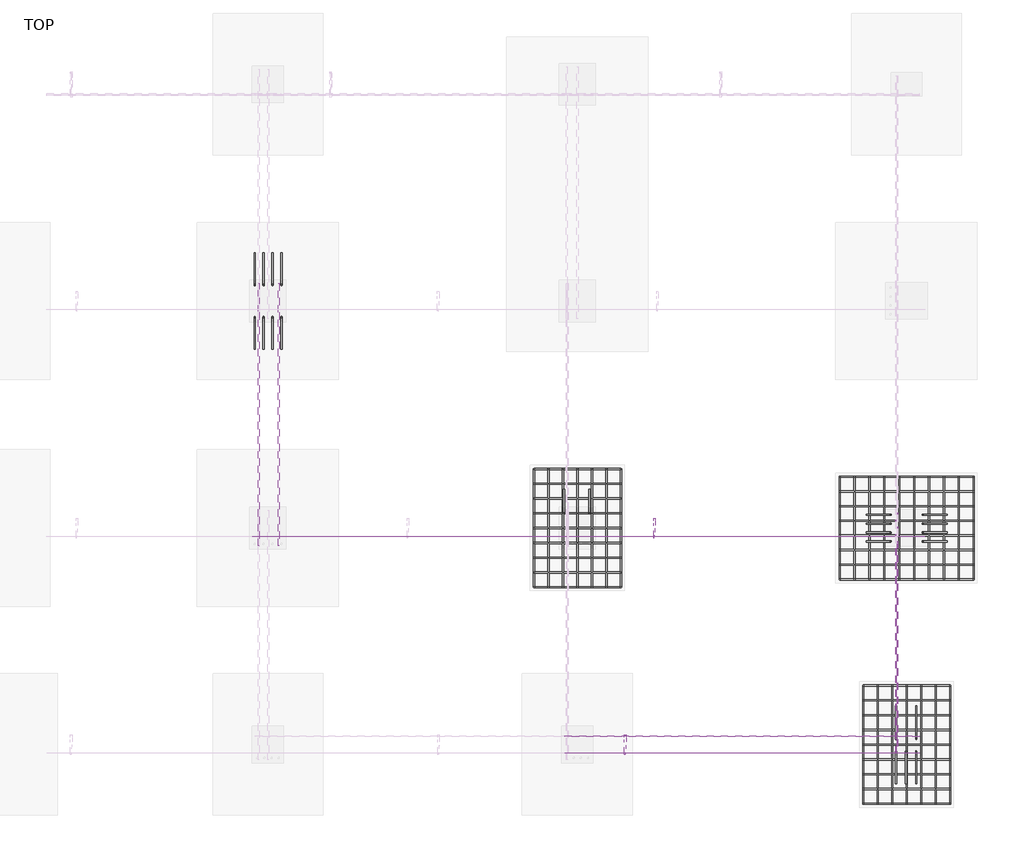
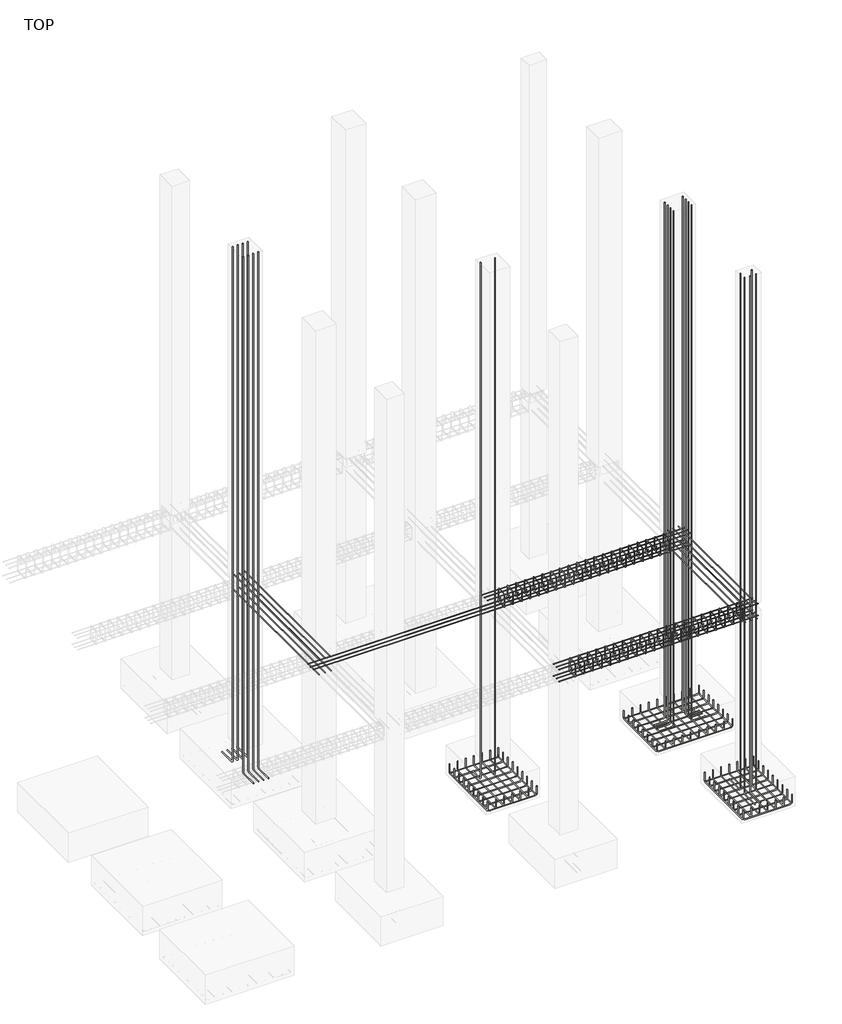
# One storey, part 6 of 8: 24 reinforcing bars.
"""IFC4 building model written with IfcOpenShell, lengths in millimetres."""

from ifc_helpers import new_model, si_unit, point, frame, origin, place, context, project, spatial, polyline, circle_curve, trimmed, segment, composite_curve, source, transform, mapped, element, save
from ifc_brep_helpers import swept_disk

model = new_model("IFC4")

# Units and contexts
model_context = context("Model", 3, world=origin())
ifc_project = project(units=[si_unit("LENGTHUNIT", "METRE", prefix="MILLI")], contexts=[model_context])

# Site, building, storey
site = spatial("IfcSite", under=ifc_project)
building = spatial("IfcBuilding", under=site)
storey = spatial("IfcBuildingStorey", under=building, Name="TOP", Elevation=0.0)

# Reinforcing bars
placement = place(None, origin())
reinforcing_bar_shape = source(origin(), model_context, "Body", "SolidModel", [
    swept_disk(composite_curve([segment(polyline([(3413.8839399, 2647.5307576, -331.0), (3413.8839399, 2647.5307576, -467.4)]), True, "CONTINUOUS"), segment(trimmed(circle_curve(frame((3413.8839399, 2677.5307576, -467.4), z_axis=(1.0, 0.0, 0.0), x_axis=(0.0, -30.0, 0.0)), 30.0), [point((3413.8839399, 2647.5307576, -467.4))], [point((3413.8839399, 2677.5307576, -497.4))], True, "CARTESIAN"), True, "CONTINUOUS"), segment(polyline([(3413.8839399, 2677.5307576, -497.4), (3413.8839399, 3764.7307576, -497.4)]), True, "CONTINUOUS"), segment(trimmed(circle_curve(frame((3413.8839399, 3764.7307576, -467.4), z_axis=(1.0, 0.0, 0.0), x_axis=(0.0, 0.0, -30.0)), 30.0), [point((3413.8839399, 3764.7307576, -497.4))], [point((3413.8839399, 3794.7307576, -467.4))], True, "CARTESIAN"), True, "CONTINUOUS"), segment(polyline([(3413.8839399, 3794.7307576, -467.4), (3413.8839399, 3794.7307576, -331.0)]), True, "CONTINUOUS")], self_intersect=False), 6.0),
])
element("IfcReinforcingBar", 1, at=placement, inside=storey, context=model_context, shape_type="MappedRepresentation", body=[
    mapped(reinforcing_bar_shape, transform((0.0, 0.0, 0.0), x_axis=(1.0, 0.0, 0.0), y_axis=(0.0, 1.0, 0.0), z_axis=(0.0, 0.0, 1.0))),
    mapped(reinforcing_bar_shape, transform((140.4, 0.0, 0.0), x_axis=(1.0, 0.0, 0.0), y_axis=(0.0, 1.0, 0.0), z_axis=(0.0, 0.0, 1.0))),
    mapped(reinforcing_bar_shape, transform((280.8, 0.0, 0.0), x_axis=(1.0, 0.0, 0.0), y_axis=(0.0, 1.0, 0.0), z_axis=(0.0, 0.0, 1.0))),
    mapped(reinforcing_bar_shape, transform((421.2, 0.0, 0.0), x_axis=(1.0, 0.0, 0.0), y_axis=(0.0, 1.0, 0.0), z_axis=(0.0, 0.0, 1.0))),
    mapped(reinforcing_bar_shape, transform((561.6, 0.0, 0.0), x_axis=(1.0, 0.0, 0.0), y_axis=(0.0, 1.0, 0.0), z_axis=(0.0, 0.0, 1.0))),
    mapped(reinforcing_bar_shape, transform((702.0, 0.0, 0.0), x_axis=(1.0, 0.0, 0.0), y_axis=(0.0, 1.0, 0.0), z_axis=(0.0, 0.0, 1.0))),
    mapped(reinforcing_bar_shape, transform((842.4, 0.0, 0.0), x_axis=(1.0, 0.0, 0.0), y_axis=(0.0, 1.0, 0.0), z_axis=(0.0, 0.0, 1.0))),
])
reinforcing_bar_2_shape = source(origin(), model_context, "Body", "SolidModel", [
    swept_disk(composite_curve([segment(polyline([(4256.2839399, 2647.5307576, -331.0), (4256.2839399, 2647.5307576, -467.4)]), True, "CONTINUOUS"), segment(trimmed(circle_curve(frame((4226.2839399, 2647.5307576, -467.4), z_axis=(0.0, 1.0, 0.0), x_axis=(30.0, 0.0, 0.0)), 30.0), [point((4256.2839399, 2647.5307576, -467.4))], [point((4226.2839399, 2647.5307576, -497.4))], True, "CARTESIAN"), True, "CONTINUOUS"), segment(polyline([(4226.2839399, 2647.5307576, -497.4), (3443.8839399, 2647.5307576, -497.4)]), True, "CONTINUOUS"), segment(trimmed(circle_curve(frame((3443.8839399, 2647.5307576, -467.4), z_axis=(0.0, 1.0, 0.0), x_axis=(0.0, 0.0, -30.0)), 30.0), [point((3443.8839399, 2647.5307576, -497.4))], [point((3413.8839399, 2647.5307576, -467.4))], True, "CARTESIAN"), True, "CONTINUOUS"), segment(polyline([(3413.8839399, 2647.5307576, -467.4), (3413.8839399, 2647.5307576, -331.0)]), True, "CONTINUOUS")], self_intersect=False), 6.0),
])
element("IfcReinforcingBar", 2, at=placement, inside=storey, context=model_context, shape_type="MappedRepresentation", body=[
    mapped(reinforcing_bar_2_shape, transform((0.0, 0.0, 0.0), x_axis=(1.0, 0.0, 0.0), y_axis=(0.0, 1.0, 0.0), z_axis=(0.0, 0.0, 1.0))),
    mapped(reinforcing_bar_2_shape, transform((0.0, 143.4, 0.0), x_axis=(1.0, 0.0, 0.0), y_axis=(0.0, 1.0, 0.0), z_axis=(0.0, 0.0, 1.0))),
    mapped(reinforcing_bar_2_shape, transform((0.0, 286.8, 0.0), x_axis=(1.0, 0.0, 0.0), y_axis=(0.0, 1.0, 0.0), z_axis=(0.0, 0.0, 1.0))),
    mapped(reinforcing_bar_2_shape, transform((0.0, 430.2, 0.0), x_axis=(1.0, 0.0, 0.0), y_axis=(0.0, 1.0, 0.0), z_axis=(0.0, 0.0, 1.0))),
    mapped(reinforcing_bar_2_shape, transform((0.0, 573.6, 0.0), x_axis=(1.0, 0.0, 0.0), y_axis=(0.0, 1.0, 0.0), z_axis=(0.0, 0.0, 1.0))),
    mapped(reinforcing_bar_2_shape, transform((0.0, 717.0, 0.0), x_axis=(1.0, 0.0, 0.0), y_axis=(0.0, 1.0, 0.0), z_axis=(0.0, 0.0, 1.0))),
    mapped(reinforcing_bar_2_shape, transform((0.0, 860.4, 0.0), x_axis=(1.0, 0.0, 0.0), y_axis=(0.0, 1.0, 0.0), z_axis=(0.0, 0.0, 1.0))),
    mapped(reinforcing_bar_2_shape, transform((0.0, 1003.8, 0.0), x_axis=(1.0, 0.0, 0.0), y_axis=(0.0, 1.0, 0.0), z_axis=(0.0, 0.0, 1.0))),
    mapped(reinforcing_bar_2_shape, transform((0.0, 1147.2, 0.0), x_axis=(1.0, 0.0, 0.0), y_axis=(0.0, 1.0, 0.0), z_axis=(0.0, 0.0, 1.0))),
])
reinforcing_bar_3_shape = source(origin(), model_context, "Body", "SolidModel", [
    swept_disk(composite_curve([segment(polyline([(7448.2839399, 1694.7307576, -331.0), (7448.2839399, 1694.7307576, -467.4)]), True, "CONTINUOUS"), segment(trimmed(circle_curve(frame((7448.2839399, 1664.7307576, -467.4), z_axis=(-1.0, 0.0, 0.0), x_axis=(0.0, 30.0, 0.0)), 30.0), [point((7448.2839399, 1694.7307576, -467.4))], [point((7448.2839399, 1664.7307576, -497.4))], True, "CARTESIAN"), True, "CONTINUOUS"), segment(polyline([(7448.2839399, 1664.7307576, -497.4), (7448.2839399, 577.5307576, -497.4)]), True, "CONTINUOUS"), segment(trimmed(circle_curve(frame((7448.2839399, 577.5307576, -467.4), z_axis=(-1.0, 0.0, 0.0), x_axis=(0.0, 0.0, -30.0)), 30.0), [point((7448.2839399, 577.5307576, -497.4))], [point((7448.2839399, 547.5307576, -467.4))], True, "CARTESIAN"), True, "CONTINUOUS"), segment(polyline([(7448.2839399, 547.5307576, -467.4), (7448.2839399, 547.5307576, -331.0)]), True, "CONTINUOUS")], self_intersect=False), 6.0),
])
element("IfcReinforcingBar", 3, at=placement, inside=storey, context=model_context, shape_type="MappedRepresentation", body=[
    mapped(reinforcing_bar_3_shape, transform((0.0, 0.0, 0.0), x_axis=(1.0, 0.0, 0.0), y_axis=(0.0, 1.0, 0.0), z_axis=(0.0, 0.0, 1.0))),
    mapped(reinforcing_bar_3_shape, transform((-140.4, 0.0, 0.0), x_axis=(1.0, 0.0, 0.0), y_axis=(0.0, 1.0, 0.0), z_axis=(0.0, 0.0, 1.0))),
    mapped(reinforcing_bar_3_shape, transform((-280.8, 0.0, 0.0), x_axis=(1.0, 0.0, 0.0), y_axis=(0.0, 1.0, 0.0), z_axis=(0.0, 0.0, 1.0))),
    mapped(reinforcing_bar_3_shape, transform((-421.2, 0.0, 0.0), x_axis=(1.0, 0.0, 0.0), y_axis=(0.0, 1.0, 0.0), z_axis=(0.0, 0.0, 1.0))),
    mapped(reinforcing_bar_3_shape, transform((-561.6, 0.0, 0.0), x_axis=(1.0, 0.0, 0.0), y_axis=(0.0, 1.0, 0.0), z_axis=(0.0, 0.0, 1.0))),
    mapped(reinforcing_bar_3_shape, transform((-702.0, 0.0, 0.0), x_axis=(1.0, 0.0, 0.0), y_axis=(0.0, 1.0, 0.0), z_axis=(0.0, 0.0, 1.0))),
    mapped(reinforcing_bar_3_shape, transform((-842.4, 0.0, 0.0), x_axis=(1.0, 0.0, 0.0), y_axis=(0.0, 1.0, 0.0), z_axis=(0.0, 0.0, 1.0))),
])
reinforcing_bar_4_shape = source(origin(), model_context, "Body", "SolidModel", [
    swept_disk(composite_curve([segment(polyline([(6605.8839399, 1694.7307576, -331.0), (6605.8839399, 1694.7307576, -467.4)]), True, "CONTINUOUS"), segment(trimmed(circle_curve(frame((6635.8839399, 1694.7307576, -467.4), z_axis=(0.0, -1.0, 0.0), x_axis=(-30.0, 0.0, 0.0)), 30.0), [point((6605.8839399, 1694.7307576, -467.4))], [point((6635.8839399, 1694.7307576, -497.4))], True, "CARTESIAN"), True, "CONTINUOUS"), segment(polyline([(6635.8839399, 1694.7307576, -497.4), (7418.2839399, 1694.7307576, -497.4)]), True, "CONTINUOUS"), segment(trimmed(circle_curve(frame((7418.2839399, 1694.7307576, -467.4), z_axis=(0.0, -1.0, 0.0), x_axis=(0.0, 0.0, -30.0)), 30.0), [point((7418.2839399, 1694.7307576, -497.4))], [point((7448.2839399, 1694.7307576, -467.4))], True, "CARTESIAN"), True, "CONTINUOUS"), segment(polyline([(7448.2839399, 1694.7307576, -467.4), (7448.2839399, 1694.7307576, -331.0)]), True, "CONTINUOUS")], self_intersect=False), 6.0),
])
element("IfcReinforcingBar", 4, at=placement, inside=storey, context=model_context, shape_type="MappedRepresentation", body=[
    mapped(reinforcing_bar_4_shape, transform((0.0, 0.0, 0.0), x_axis=(1.0, 0.0, 0.0), y_axis=(0.0, 1.0, 0.0), z_axis=(0.0, 0.0, 1.0))),
    mapped(reinforcing_bar_4_shape, transform((0.0, -143.4, 0.0), x_axis=(1.0, 0.0, 0.0), y_axis=(0.0, 1.0, 0.0), z_axis=(0.0, 0.0, 1.0))),
    mapped(reinforcing_bar_4_shape, transform((0.0, -286.8, 0.0), x_axis=(1.0, 0.0, 0.0), y_axis=(0.0, 1.0, 0.0), z_axis=(0.0, 0.0, 1.0))),
    mapped(reinforcing_bar_4_shape, transform((0.0, -430.2, 0.0), x_axis=(1.0, 0.0, 0.0), y_axis=(0.0, 1.0, 0.0), z_axis=(0.0, 0.0, 1.0))),
    mapped(reinforcing_bar_4_shape, transform((0.0, -573.6, 0.0), x_axis=(1.0, 0.0, 0.0), y_axis=(0.0, 1.0, 0.0), z_axis=(0.0, 0.0, 1.0))),
    mapped(reinforcing_bar_4_shape, transform((0.0, -717.0, 0.0), x_axis=(1.0, 0.0, 0.0), y_axis=(0.0, 1.0, 0.0), z_axis=(0.0, 0.0, 1.0))),
    mapped(reinforcing_bar_4_shape, transform((0.0, -860.4, 0.0), x_axis=(1.0, 0.0, 0.0), y_axis=(0.0, 1.0, 0.0), z_axis=(0.0, 0.0, 1.0))),
    mapped(reinforcing_bar_4_shape, transform((0.0, -1003.8, 0.0), x_axis=(1.0, 0.0, 0.0), y_axis=(0.0, 1.0, 0.0), z_axis=(0.0, 0.0, 1.0))),
    mapped(reinforcing_bar_4_shape, transform((0.0, -1147.2, 0.0), x_axis=(1.0, 0.0, 0.0), y_axis=(0.0, 1.0, 0.0), z_axis=(0.0, 0.0, 1.0))),
])
reinforcing_bar_5_shape = source(origin(), model_context, "Body", "SolidModel", [
    swept_disk(composite_curve([segment(polyline([(6922.6839399, 1177.1568407, 8968.464), (6922.6839399, 1177.1568407, -415.886)]), True, "CONTINUOUS"), segment(trimmed(circle_curve(frame((6922.6839399, 1207.1568407, -415.886), z_axis=(1.0, 0.0, 0.0), x_axis=(0.0, -30.0, 0.0)), 30.0), [point((6922.6839399, 1177.1568407, -415.886))], [point((6922.6839399, 1207.1568407, -445.886))], True, "CARTESIAN"), True, "CONTINUOUS"), segment(polyline([(6922.6839399, 1207.1568407, -445.886), (6922.6839399, 1500.2307576, -445.886)]), True, "CONTINUOUS")], self_intersect=False), 6.0),
])
element("IfcReinforcingBar", 5, at=placement, inside=storey, context=model_context, shape_type="MappedRepresentation", body=[
    mapped(reinforcing_bar_5_shape, transform((0.0, 0.0, 0.0), x_axis=(1.0, 0.0, 0.0), y_axis=(0.0, 1.0, 0.0), z_axis=(0.0, 0.0, 1.0))),
    mapped(reinforcing_bar_5_shape, transform((195.9681172, 0.0, 0.0), x_axis=(1.0, 0.0, 0.0), y_axis=(0.0, 1.0, 0.0), z_axis=(0.0, 0.0, 1.0))),
])
reinforcing_bar_6_shape = source(origin(), model_context, "Body", "SolidModel", [
    swept_disk(composite_curve([segment(polyline([(7118.6520571, 1054.8307576, 8968.464), (7118.6520571, 1054.8307576, -415.886)]), True, "CONTINUOUS"), segment(trimmed(circle_curve(frame((7118.6520571, 1024.8307576, -415.886), z_axis=(-1.0, 0.0, 0.0), x_axis=(0.0, 30.0, 0.0)), 30.0), [point((7118.6520571, 1054.8307576, -415.886))], [point((7118.6520571, 1024.8307576, -445.886))], True, "CARTESIAN"), True, "CONTINUOUS"), segment(polyline([(7118.6520571, 1024.8307576, -445.886), (7118.6520571, 742.0307576, -445.886)]), True, "CONTINUOUS")], self_intersect=False), 6.0),
])
element("IfcReinforcingBar", 6, at=placement, inside=storey, context=model_context, shape_type="MappedRepresentation", body=[
    mapped(reinforcing_bar_6_shape, transform((0.0, 0.0, 0.0), x_axis=(1.0, 0.0, 0.0), y_axis=(0.0, 1.0, 0.0), z_axis=(0.0, 0.0, 1.0))),
    mapped(reinforcing_bar_6_shape, transform((-97.9840586, 0.0, 0.0), x_axis=(1.0, 0.0, 0.0), y_axis=(0.0, 1.0, 0.0), z_axis=(0.0, 0.0, 1.0))),
    mapped(reinforcing_bar_6_shape, transform((-195.9681172, 0.0, 0.0), x_axis=(1.0, 0.0, 0.0), y_axis=(0.0, 1.0, 0.0), z_axis=(0.0, 0.0, 1.0))),
])
reinforcing_bar_7_shape = source(origin(), model_context, "Body", "SolidModel", [
    swept_disk(composite_curve([segment(polyline([(3705.2331399, 3366.0060407, 8968.464), (3705.2331399, 3366.0060407, -415.886)]), True, "CONTINUOUS"), segment(trimmed(circle_curve(frame((3705.2331399, 3396.0060407, -415.886), z_axis=(1.0, 0.0, 0.0), x_axis=(0.0, -30.0, 0.0)), 30.0), [point((3705.2331399, 3366.0060407, -415.886))], [point((3705.2331399, 3396.0060407, -445.886))], True, "CARTESIAN"), True, "CONTINUOUS"), segment(polyline([(3705.2331399, 3396.0060407, -445.886), (3705.2331399, 3600.2307576, -445.886)]), True, "CONTINUOUS")], self_intersect=False), 6.0),
])
element("IfcReinforcingBar", 7, at=placement, inside=storey, context=model_context, shape_type="MappedRepresentation", body=[
    mapped(reinforcing_bar_7_shape, transform((0.0, 0.0, 0.0), x_axis=(1.0, 0.0, 0.0), y_axis=(0.0, 1.0, 0.0), z_axis=(0.0, 0.0, 1.0))),
    mapped(reinforcing_bar_7_shape, transform((246.8697172, 0.0, 0.0), x_axis=(1.0, 0.0, 0.0), y_axis=(0.0, 1.0, 0.0), z_axis=(0.0, 0.0, 1.0))),
])
reinforcing_bar_8_shape = source(origin(), model_context, "Body", "SolidModel", [
    swept_disk(composite_curve([segment(polyline([(6377.2839399, 3718.5307576, -351.0), (6377.2839399, 3718.5307576, -467.4)]), True, "CONTINUOUS"), segment(trimmed(circle_curve(frame((6407.2839399, 3718.5307576, -467.4), z_axis=(0.0, -1.0, 0.0), x_axis=(-30.0, 0.0, 0.0)), 30.0), [point((6377.2839399, 3718.5307576, -467.4))], [point((6407.2839399, 3718.5307576, -497.4))], True, "CARTESIAN"), True, "CONTINUOUS"), segment(polyline([(6407.2839399, 3718.5307576, -497.4), (7646.8839399, 3718.5307576, -497.4)]), True, "CONTINUOUS"), segment(trimmed(circle_curve(frame((7646.8839399, 3718.5307576, -467.4), z_axis=(0.0, -1.0, 0.0), x_axis=(0.0, 0.0, -30.0)), 30.0), [point((7646.8839399, 3718.5307576, -497.4))], [point((7676.8839399, 3718.5307576, -467.4))], True, "CARTESIAN"), True, "CONTINUOUS"), segment(polyline([(7676.8839399, 3718.5307576, -467.4), (7676.8839399, 3718.5307576, -351.0)]), True, "CONTINUOUS")], self_intersect=False), 6.0),
])
element("IfcReinforcingBar", 8, at=placement, inside=storey, context=model_context, shape_type="MappedRepresentation", body=[
    mapped(reinforcing_bar_8_shape, transform((0.0, 0.0, 0.0), x_axis=(1.0, 0.0, 0.0), y_axis=(0.0, 1.0, 0.0), z_axis=(0.0, 0.0, 1.0))),
    mapped(reinforcing_bar_8_shape, transform((0.0, -142.1142857, 0.0), x_axis=(1.0, 0.0, 0.0), y_axis=(0.0, 1.0, 0.0), z_axis=(0.0, 0.0, 1.0))),
    mapped(reinforcing_bar_8_shape, transform((0.0, -284.2285714, 0.0), x_axis=(1.0, 0.0, 0.0), y_axis=(0.0, 1.0, 0.0), z_axis=(0.0, 0.0, 1.0))),
    mapped(reinforcing_bar_8_shape, transform((0.0, -426.3428571, 0.0), x_axis=(1.0, 0.0, 0.0), y_axis=(0.0, 1.0, 0.0), z_axis=(0.0, 0.0, 1.0))),
    mapped(reinforcing_bar_8_shape, transform((0.0, -568.4571429, 0.0), x_axis=(1.0, 0.0, 0.0), y_axis=(0.0, 1.0, 0.0), z_axis=(0.0, 0.0, 1.0))),
    mapped(reinforcing_bar_8_shape, transform((0.0, -710.5714286, 0.0), x_axis=(1.0, 0.0, 0.0), y_axis=(0.0, 1.0, 0.0), z_axis=(0.0, 0.0, 1.0))),
    mapped(reinforcing_bar_8_shape, transform((0.0, -852.6857143, 0.0), x_axis=(1.0, 0.0, 0.0), y_axis=(0.0, 1.0, 0.0), z_axis=(0.0, 0.0, 1.0))),
    mapped(reinforcing_bar_8_shape, transform((0.0, -994.8, 0.0), x_axis=(1.0, 0.0, 0.0), y_axis=(0.0, 1.0, 0.0), z_axis=(0.0, 0.0, 1.0))),
])
reinforcing_bar_9_shape = source(origin(), model_context, "Body", "SolidModel", [
    swept_disk(composite_curve([segment(polyline([(6377.2839399, 2723.7307576, -351.0), (6377.2839399, 2723.7307576, -467.4)]), True, "CONTINUOUS"), segment(trimmed(circle_curve(frame((6377.2839399, 2753.7307576, -467.4), z_axis=(1.0, 0.0, 0.0), x_axis=(0.0, -30.0, 0.0)), 30.0), [point((6377.2839399, 2723.7307576, -467.4))], [point((6377.2839399, 2753.7307576, -497.4))], True, "CARTESIAN"), True, "CONTINUOUS"), segment(polyline([(6377.2839399, 2753.7307576, -497.4), (6377.2839399, 3688.5307576, -497.4)]), True, "CONTINUOUS"), segment(trimmed(circle_curve(frame((6377.2839399, 3688.5307576, -467.4), z_axis=(1.0, 0.0, 0.0), x_axis=(0.0, 0.0, -30.0)), 30.0), [point((6377.2839399, 3688.5307576, -497.4))], [point((6377.2839399, 3718.5307576, -467.4))], True, "CARTESIAN"), True, "CONTINUOUS"), segment(polyline([(6377.2839399, 3718.5307576, -467.4), (6377.2839399, 3718.5307576, -351.0)]), True, "CONTINUOUS")], self_intersect=False), 6.0),
])
element("IfcReinforcingBar", 9, at=placement, inside=storey, context=model_context, shape_type="MappedRepresentation", body=[
    mapped(reinforcing_bar_9_shape, transform((0.0, 0.0, 0.0), x_axis=(1.0, 0.0, 0.0), y_axis=(0.0, 1.0, 0.0), z_axis=(0.0, 0.0, 1.0))),
    mapped(reinforcing_bar_9_shape, transform((144.4, 0.0, 0.0), x_axis=(1.0, 0.0, 0.0), y_axis=(0.0, 1.0, 0.0), z_axis=(0.0, 0.0, 1.0))),
    mapped(reinforcing_bar_9_shape, transform((288.8, 0.0, 0.0), x_axis=(1.0, 0.0, 0.0), y_axis=(0.0, 1.0, 0.0), z_axis=(0.0, 0.0, 1.0))),
    mapped(reinforcing_bar_9_shape, transform((433.2, 0.0, 0.0), x_axis=(1.0, 0.0, 0.0), y_axis=(0.0, 1.0, 0.0), z_axis=(0.0, 0.0, 1.0))),
    mapped(reinforcing_bar_9_shape, transform((577.6, 0.0, 0.0), x_axis=(1.0, 0.0, 0.0), y_axis=(0.0, 1.0, 0.0), z_axis=(0.0, 0.0, 1.0))),
    mapped(reinforcing_bar_9_shape, transform((722.0, 0.0, 0.0), x_axis=(1.0, 0.0, 0.0), y_axis=(0.0, 1.0, 0.0), z_axis=(0.0, 0.0, 1.0))),
    mapped(reinforcing_bar_9_shape, transform((866.4, 0.0, 0.0), x_axis=(1.0, 0.0, 0.0), y_axis=(0.0, 1.0, 0.0), z_axis=(0.0, 0.0, 1.0))),
    mapped(reinforcing_bar_9_shape, transform((1010.8, 0.0, 0.0), x_axis=(1.0, 0.0, 0.0), y_axis=(0.0, 1.0, 0.0), z_axis=(0.0, 0.0, 1.0))),
    mapped(reinforcing_bar_9_shape, transform((1155.2, 0.0, 0.0), x_axis=(1.0, 0.0, 0.0), y_axis=(0.0, 1.0, 0.0), z_axis=(0.0, 0.0, 1.0))),
    mapped(reinforcing_bar_9_shape, transform((1299.6, 0.0, 0.0), x_axis=(1.0, 0.0, 0.0), y_axis=(0.0, 1.0, 0.0), z_axis=(0.0, 0.0, 1.0))),
])
reinforcing_bar_10_shape = source(origin(), model_context, "Body", "SolidModel", [
    swept_disk(composite_curve([segment(polyline([(6871.9347399, 3091.2799576, 8968.464), (6871.9347399, 3091.2799576, -403.186)]), True, "CONTINUOUS"), segment(trimmed(circle_curve(frame((6841.9347399, 3091.2799576, -403.186), z_axis=(0.0, 1.0, 0.0), x_axis=(30.0, 0.0, 0.0)), 30.0), [point((6871.9347399, 3091.2799576, -403.186))], [point((6841.9347399, 3091.2799576, -433.186))], True, "CARTESIAN"), True, "CONTINUOUS"), segment(polyline([(6841.9347399, 3091.2799576, -433.186), (6635.3347399, 3091.2799576, -433.186)]), True, "CONTINUOUS")], self_intersect=False), 6.0),
])
element("IfcReinforcingBar", 10, at=placement, inside=storey, context=model_context, shape_type="MappedRepresentation", body=[
    mapped(reinforcing_bar_10_shape, transform((0.0, 0.0, 0.0), x_axis=(1.0, 0.0, 0.0), y_axis=(0.0, 1.0, 0.0), z_axis=(0.0, 0.0, 1.0))),
    mapped(reinforcing_bar_10_shape, transform((0.0, 86.5672, 0.0), x_axis=(1.0, 0.0, 0.0), y_axis=(0.0, 1.0, 0.0), z_axis=(0.0, 0.0, 1.0))),
    mapped(reinforcing_bar_10_shape, transform((0.0, 173.1344, 0.0), x_axis=(1.0, 0.0, 0.0), y_axis=(0.0, 1.0, 0.0), z_axis=(0.0, 0.0, 1.0))),
    mapped(reinforcing_bar_10_shape, transform((0.0, 259.7016, 0.0), x_axis=(1.0, 0.0, 0.0), y_axis=(0.0, 1.0, 0.0), z_axis=(0.0, 0.0, 1.0))),
])
reinforcing_bar_11_shape = source(origin(), model_context, "Body", "SolidModel", [
    swept_disk(composite_curve([segment(polyline([(7182.2331399, 3350.9815576, 8968.464), (7182.2331399, 3350.9815576, -409.536)]), True, "CONTINUOUS"), segment(trimmed(circle_curve(frame((7212.2331399, 3350.9815576, -409.536), z_axis=(0.0, -1.0, 0.0), x_axis=(-30.0, 0.0, 0.0)), 30.0), [point((7182.2331399, 3350.9815576, -409.536))], [point((7212.2331399, 3350.9815576, -439.536))], True, "CARTESIAN"), True, "CONTINUOUS"), segment(polyline([(7212.2331399, 3350.9815576, -439.536), (7418.8331399, 3350.9815576, -439.536)]), True, "CONTINUOUS")], self_intersect=False), 6.0),
])
element("IfcReinforcingBar", 11, at=placement, inside=storey, context=model_context, shape_type="MappedRepresentation", body=[
    mapped(reinforcing_bar_11_shape, transform((0.0, 0.0, 0.0), x_axis=(1.0, 0.0, 0.0), y_axis=(0.0, 1.0, 0.0), z_axis=(0.0, 0.0, 1.0))),
    mapped(reinforcing_bar_11_shape, transform((0.0, -86.5672, 0.0), x_axis=(1.0, 0.0, 0.0), y_axis=(0.0, 1.0, 0.0), z_axis=(0.0, 0.0, 1.0))),
    mapped(reinforcing_bar_11_shape, transform((0.0, -173.1344, 0.0), x_axis=(1.0, 0.0, 0.0), y_axis=(0.0, 1.0, 0.0), z_axis=(0.0, 0.0, 1.0))),
    mapped(reinforcing_bar_11_shape, transform((0.0, -259.7016, 0.0), x_axis=(1.0, 0.0, 0.0), y_axis=(0.0, 1.0, 0.0), z_axis=(0.0, 0.0, 1.0))),
])
reinforcing_bar_12_shape = source(origin(), model_context, "Body", "SolidModel", [
    swept_disk(composite_curve([segment(polyline([(705.2331399, 5577.0799576, 8968.464), (705.2331399, 5577.0799576, -403.186)]), True, "CONTINUOUS"), segment(trimmed(circle_curve(frame((705.2331399, 5607.0799576, -403.186), z_axis=(1.0, 0.0, 0.0), x_axis=(0.0, -30.0, 0.0)), 30.0), [point((705.2331399, 5577.0799576, -403.186))], [point((705.2331399, 5607.0799576, -433.186))], True, "CARTESIAN"), True, "CONTINUOUS"), segment(polyline([(705.2331399, 5607.0799576, -433.186), (705.2331399, 5889.8799576, -433.186)]), True, "CONTINUOUS")], self_intersect=False), 6.0),
])
element("IfcReinforcingBar", 12, at=placement, inside=storey, context=model_context, shape_type="MappedRepresentation", body=[
    mapped(reinforcing_bar_12_shape, transform((0.0, 0.0, 0.0), x_axis=(1.0, 0.0, 0.0), y_axis=(0.0, 1.0, 0.0), z_axis=(0.0, 0.0, 1.0))),
    mapped(reinforcing_bar_12_shape, transform((86.5672, 0.0, 0.0), x_axis=(1.0, 0.0, 0.0), y_axis=(0.0, 1.0, 0.0), z_axis=(0.0, 0.0, 1.0))),
    mapped(reinforcing_bar_12_shape, transform((173.1344, 0.0, 0.0), x_axis=(1.0, 0.0, 0.0), y_axis=(0.0, 1.0, 0.0), z_axis=(0.0, 0.0, 1.0))),
    mapped(reinforcing_bar_12_shape, transform((259.7016, 0.0, 0.0), x_axis=(1.0, 0.0, 0.0), y_axis=(0.0, 1.0, 0.0), z_axis=(0.0, 0.0, 1.0))),
])
reinforcing_bar_13_shape = source(origin(), model_context, "Body", "SolidModel", [
    swept_disk(composite_curve([segment(polyline([(964.9347399, 5266.7815576, 8968.464), (964.9347399, 5266.7815576, -409.536)]), True, "CONTINUOUS"), segment(trimmed(circle_curve(frame((964.9347399, 5236.7815576, -409.536), z_axis=(-1.0, 0.0, 0.0), x_axis=(0.0, 30.0, 0.0)), 30.0), [point((964.9347399, 5266.7815576, -409.536))], [point((964.9347399, 5236.7815576, -439.536))], True, "CARTESIAN"), True, "CONTINUOUS"), segment(polyline([(964.9347399, 5236.7815576, -439.536), (964.9347399, 4953.9815576, -439.536)]), True, "CONTINUOUS")], self_intersect=False), 6.0),
])
element("IfcReinforcingBar", 13, at=placement, inside=storey, context=model_context, shape_type="MappedRepresentation", body=[
    mapped(reinforcing_bar_13_shape, transform((0.0, 0.0, 0.0), x_axis=(1.0, 0.0, 0.0), y_axis=(0.0, 1.0, 0.0), z_axis=(0.0, 0.0, 1.0))),
    mapped(reinforcing_bar_13_shape, transform((-86.5672, 0.0, 0.0), x_axis=(1.0, 0.0, 0.0), y_axis=(0.0, 1.0, 0.0), z_axis=(0.0, 0.0, 1.0))),
    mapped(reinforcing_bar_13_shape, transform((-173.1344, 0.0, 0.0), x_axis=(1.0, 0.0, 0.0), y_axis=(0.0, 1.0, 0.0), z_axis=(0.0, 0.0, 1.0))),
    mapped(reinforcing_bar_13_shape, transform((-259.7016, 0.0, 0.0), x_axis=(1.0, 0.0, 0.0), y_axis=(0.0, 1.0, 0.0), z_axis=(0.0, 0.0, 1.0))),
])
reinforcing_bar_14_shape = source(origin(), model_context, "Body", "SolidModel", [
    swept_disk(composite_curve([segment(polyline([(732.0773382, 5595.0799576, 2693.6917983), (732.0773382, 3047.9815576, 2693.6917983)]), True, "CONTINUOUS")], self_intersect=False), 5.0),
])
element("IfcReinforcingBar", 14, at=placement, inside=storey, context=model_context, shape_type="MappedRepresentation", body=[
    mapped(reinforcing_bar_14_shape, transform((0.0, 0.0, 0.0), x_axis=(1.0, 0.0, 0.0), y_axis=(0.0, 1.0, 0.0), z_axis=(0.0, 0.0, 1.0))),
    mapped(reinforcing_bar_14_shape, transform((103.0066017, 0.0, 0.0), x_axis=(1.0, 0.0, 0.0), y_axis=(0.0, 1.0, 0.0), z_axis=(0.0, 0.0, 1.0))),
    mapped(reinforcing_bar_14_shape, transform((206.0132034, 0.0, 0.0), x_axis=(1.0, 0.0, 0.0), y_axis=(0.0, 1.0, 0.0), z_axis=(0.0, 0.0, 1.0))),
])
reinforcing_bar_15_shape = source(origin(), model_context, "Body", "SolidModel", [
    swept_disk(composite_curve([segment(polyline([(742.6839399, 3047.9815576, 2955.0), (742.6839399, 5595.0799576, 2955.0)]), True, "CONTINUOUS")], self_intersect=False), 5.0),
])
element("IfcReinforcingBar", 15, at=placement, inside=storey, context=model_context, shape_type="MappedRepresentation", body=[
    mapped(reinforcing_bar_15_shape, transform((0.0, 0.0, 0.0), x_axis=(1.0, 0.0, 0.0), y_axis=(0.0, 1.0, 0.0), z_axis=(0.0, 0.0, 1.0))),
    mapped(reinforcing_bar_15_shape, transform((92.4, 0.0, 0.0), x_axis=(1.0, 0.0, 0.0), y_axis=(0.0, 1.0, 0.0), z_axis=(0.0, 0.0, 1.0))),
    mapped(reinforcing_bar_15_shape, transform((184.8, 0.0, 0.0), x_axis=(1.0, 0.0, 0.0), y_axis=(0.0, 1.0, 0.0), z_axis=(0.0, 0.0, 1.0))),
])
reinforcing_bar_16_shape = source(origin(), model_context, "Body", "SolidModel", [
    swept_disk(composite_curve([segment(polyline([(6924.0773382, 3368.9815576, 2693.6917983), (6924.0773382, 1036.8307576, 2693.6917983)]), True, "CONTINUOUS")], self_intersect=False), 5.0),
])
element("IfcReinforcingBar", 16, at=placement, inside=storey, context=model_context, shape_type="MappedRepresentation", body=[
    mapped(reinforcing_bar_16_shape, transform((0.0, 0.0, 0.0), x_axis=(1.0, 0.0, 0.0), y_axis=(0.0, 1.0, 0.0), z_axis=(0.0, 0.0, 1.0))),
    mapped(reinforcing_bar_16_shape, transform((103.0066017, 0.0, 0.0), x_axis=(1.0, 0.0, 0.0), y_axis=(0.0, 1.0, 0.0), z_axis=(0.0, 0.0, 1.0))),
    mapped(reinforcing_bar_16_shape, transform((206.0132034, 0.0, 0.0), x_axis=(1.0, 0.0, 0.0), y_axis=(0.0, 1.0, 0.0), z_axis=(0.0, 0.0, 1.0))),
])
reinforcing_bar_17_shape = source(origin(), model_context, "Body", "SolidModel", [
    swept_disk(composite_curve([segment(polyline([(6934.6839399, 1036.8307576, 2955.0), (6934.6839399, 3368.9815576, 2955.0)]), True, "CONTINUOUS")], self_intersect=False), 5.0),
])
element("IfcReinforcingBar", 17, at=placement, inside=storey, context=model_context, shape_type="MappedRepresentation", body=[
    mapped(reinforcing_bar_17_shape, transform((0.0, 0.0, 0.0), x_axis=(1.0, 0.0, 0.0), y_axis=(0.0, 1.0, 0.0), z_axis=(0.0, 0.0, 1.0))),
    mapped(reinforcing_bar_17_shape, transform((92.4, 0.0, 0.0), x_axis=(1.0, 0.0, 0.0), y_axis=(0.0, 1.0, 0.0), z_axis=(0.0, 0.0, 1.0))),
    mapped(reinforcing_bar_17_shape, transform((184.8, 0.0, 0.0), x_axis=(1.0, 0.0, 0.0), y_axis=(0.0, 1.0, 0.0), z_axis=(0.0, 0.0, 1.0))),
])
reinforcing_bar_18_shape = source(origin(), model_context, "Body", "SolidModel", [
    swept_disk(composite_curve([segment(polyline([(3982.9347399, 3302.565239, 2740.7147186), (687.2331399, 3302.565239, 2740.7147186)]), True, "CONTINUOUS")], self_intersect=False), 4.0),
])
element("IfcReinforcingBar", 18, at=placement, inside=storey, context=model_context, shape_type="MappedRepresentation", body=[
    mapped(reinforcing_bar_18_shape, transform((0.0, 0.0, 0.0), x_axis=(1.0, 0.0, 0.0), y_axis=(0.0, 1.0, 0.0), z_axis=(0.0, 0.0, 1.0))),
    mapped(reinforcing_bar_18_shape, transform((0.0, -81.4344814, 0.0), x_axis=(1.0, 0.0, 0.0), y_axis=(0.0, 1.0, 0.0), z_axis=(0.0, 0.0, 1.0))),
    mapped(reinforcing_bar_18_shape, transform((0.0, -162.8689627, 0.0), x_axis=(1.0, 0.0, 0.0), y_axis=(0.0, 1.0, 0.0), z_axis=(0.0, 0.0, 1.0))),
])
reinforcing_bar_19_shape = source(origin(), model_context, "Body", "SolidModel", [
    swept_disk(composite_curve([segment(polyline([(6870.8331399, 1143.8753761, 2827.6888527), (6870.8331399, 1208.2220932, 2763.3421356)]), True, "CONTINUOUS"), segment(trimmed(circle_curve(frame((6870.8331399, 1194.0799576, 2749.2), z_axis=(-1.0, 0.0, 0.0), x_axis=(0.0, 14.142135600000074, 14.142135600000074)), 20.0), [point((6870.8331399, 1208.2220932, 2763.3421356))], [point((6870.8331399, 1194.0799576, 2729.2))], True, "CARTESIAN"), True, "CONTINUOUS"), segment(polyline([(6870.8331399, 1194.0799576, 2729.2), (6870.8331399, 1048.1815576, 2729.2)]), True, "CONTINUOUS"), segment(trimmed(circle_curve(frame((6870.8331399, 1048.1815576, 2749.2), z_axis=(-1.0, 0.0, 0.0), x_axis=(0.0, 0.0, -20.0)), 20.0), [point((6870.8331399, 1048.1815576, 2729.2))], [point((6870.8331399, 1028.1815576, 2749.2))], True, "CARTESIAN"), True, "CONTINUOUS"), segment(polyline([(6870.8331399, 1028.1815576, 2749.2), (6870.8331399, 1028.1815576, 2946.0)]), True, "CONTINUOUS"), segment(trimmed(circle_curve(frame((6871.6930293, 1048.1630638, 2946.0), z_axis=(-0.9990753104108542, 0.04299446624224496, 0.0), x_axis=(-0.8598893999997017, -19.981506200000013, 0.0)), 20.0), [point((6870.8331399, 1028.1815576, 2946.0))], [point((6871.6930293, 1048.1630638, 2966.0))], True, "CARTESIAN"), True, "CONTINUOUS"), segment(polyline([(6871.6930293, 1048.1630638, 2966.0), (6877.9732506, 1194.0984514, 2966.0)]), True, "CONTINUOUS"), segment(trimmed(circle_curve(frame((6877.9732506, 1194.0984514, 2946.0), z_axis=(-0.9990753104108542, 0.04299446624224496, 0.0), x_axis=(0.0, 0.0, 20.0)), 20.0), [point((6877.9732506, 1194.0984514, 2966.0))], [point((6878.8331399, 1214.0799576, 2946.0))], True, "CARTESIAN"), True, "CONTINUOUS"), segment(polyline([(6878.8331399, 1214.0799576, 2946.0), (6878.8331399, 1214.0799576, 2749.2)]), True, "CONTINUOUS"), segment(trimmed(circle_curve(frame((6878.8331399, 1194.0799576, 2749.2), z_axis=(-1.0, 0.0, 0.0), x_axis=(0.0, 20.0, 0.0)), 20.0), [point((6878.8331399, 1214.0799576, 2749.2))], [point((6878.8331399, 1179.937822, 2735.0578644))], True, "CARTESIAN"), True, "CONTINUOUS"), segment(polyline([(6878.8331399, 1179.937822, 2735.0578644), (6878.8331399, 1115.5911049, 2799.4045815)]), True, "CONTINUOUS")], self_intersect=False), 4.0),
])
element("IfcReinforcingBar", 19, at=placement, inside=storey, context=model_context, shape_type="MappedRepresentation", body=[
    mapped(reinforcing_bar_19_shape, transform((0.0, 0.0, 0.0), x_axis=(1.0, 0.0, 0.0), y_axis=(0.0, 1.0, 0.0), z_axis=(0.0, 0.0, 1.0))),
    mapped(reinforcing_bar_19_shape, transform((-151.5446947, 0.0, 0.0), x_axis=(1.0, 0.0, 0.0), y_axis=(0.0, 1.0, 0.0), z_axis=(0.0, 0.0, 1.0))),
    mapped(reinforcing_bar_19_shape, transform((-303.0893895, 0.0, 0.0), x_axis=(1.0, 0.0, 0.0), y_axis=(0.0, 1.0, 0.0), z_axis=(0.0, 0.0, 1.0))),
    mapped(reinforcing_bar_19_shape, transform((-454.6340842, 0.0, 0.0), x_axis=(1.0, 0.0, 0.0), y_axis=(0.0, 1.0, 0.0), z_axis=(0.0, 0.0, 1.0))),
    mapped(reinforcing_bar_19_shape, transform((-606.1787789, 0.0, 0.0), x_axis=(1.0, 0.0, 0.0), y_axis=(0.0, 1.0, 0.0), z_axis=(0.0, 0.0, 1.0))),
    mapped(reinforcing_bar_19_shape, transform((-757.7234737, 0.0, 0.0), x_axis=(1.0, 0.0, 0.0), y_axis=(0.0, 1.0, 0.0), z_axis=(0.0, 0.0, 1.0))),
    mapped(reinforcing_bar_19_shape, transform((-909.2681684, 0.0, 0.0), x_axis=(1.0, 0.0, 0.0), y_axis=(0.0, 1.0, 0.0), z_axis=(0.0, 0.0, 1.0))),
    mapped(reinforcing_bar_19_shape, transform((-1060.8128632, 0.0, 0.0), x_axis=(1.0, 0.0, 0.0), y_axis=(0.0, 1.0, 0.0), z_axis=(0.0, 0.0, 1.0))),
    mapped(reinforcing_bar_19_shape, transform((-1212.3575579, 0.0, 0.0), x_axis=(1.0, 0.0, 0.0), y_axis=(0.0, 1.0, 0.0), z_axis=(0.0, 0.0, 1.0))),
    mapped(reinforcing_bar_19_shape, transform((-1363.9022526, 0.0, 0.0), x_axis=(1.0, 0.0, 0.0), y_axis=(0.0, 1.0, 0.0), z_axis=(0.0, 0.0, 1.0))),
    mapped(reinforcing_bar_19_shape, transform((-1515.4469474, 0.0, 0.0), x_axis=(1.0, 0.0, 0.0), y_axis=(0.0, 1.0, 0.0), z_axis=(0.0, 0.0, 1.0))),
    mapped(reinforcing_bar_19_shape, transform((-1666.9916421, 0.0, 0.0), x_axis=(1.0, 0.0, 0.0), y_axis=(0.0, 1.0, 0.0), z_axis=(0.0, 0.0, 1.0))),
    mapped(reinforcing_bar_19_shape, transform((-1818.5363368, 0.0, 0.0), x_axis=(1.0, 0.0, 0.0), y_axis=(0.0, 1.0, 0.0), z_axis=(0.0, 0.0, 1.0))),
    mapped(reinforcing_bar_19_shape, transform((-1970.0810316, 0.0, 0.0), x_axis=(1.0, 0.0, 0.0), y_axis=(0.0, 1.0, 0.0), z_axis=(0.0, 0.0, 1.0))),
    mapped(reinforcing_bar_19_shape, transform((-2121.6257263, 0.0, 0.0), x_axis=(1.0, 0.0, 0.0), y_axis=(0.0, 1.0, 0.0), z_axis=(0.0, 0.0, 1.0))),
    mapped(reinforcing_bar_19_shape, transform((-2273.1704211, 0.0, 0.0), x_axis=(1.0, 0.0, 0.0), y_axis=(0.0, 1.0, 0.0), z_axis=(0.0, 0.0, 1.0))),
    mapped(reinforcing_bar_19_shape, transform((-2424.7151158, 0.0, 0.0), x_axis=(1.0, 0.0, 0.0), y_axis=(0.0, 1.0, 0.0), z_axis=(0.0, 0.0, 1.0))),
    mapped(reinforcing_bar_19_shape, transform((-2576.2598105, 0.0, 0.0), x_axis=(1.0, 0.0, 0.0), y_axis=(0.0, 1.0, 0.0), z_axis=(0.0, 0.0, 1.0))),
    mapped(reinforcing_bar_19_shape, transform((-2727.8045053, 0.0, 0.0), x_axis=(1.0, 0.0, 0.0), y_axis=(0.0, 1.0, 0.0), z_axis=(0.0, 0.0, 1.0))),
    mapped(reinforcing_bar_19_shape, transform((-2879.3492, 0.0, 0.0), x_axis=(1.0, 0.0, 0.0), y_axis=(0.0, 1.0, 0.0), z_axis=(0.0, 0.0, 1.0))),
])
reinforcing_bar_20_shape = source(origin(), model_context, "Body", "SolidModel", [
    swept_disk(composite_curve([segment(polyline([(7149.4839399, 1039.6962762, 2954.4852814), (3712.6839399, 1039.6962762, 2954.4852814)]), True, "CONTINUOUS")], self_intersect=False), 4.0),
])
element("IfcReinforcingBar", 20, at=placement, inside=storey, context=model_context, shape_type="MappedRepresentation", body=[
    mapped(reinforcing_bar_20_shape, transform((0.0, 0.0, 0.0), x_axis=(1.0, 0.0, 0.0), y_axis=(0.0, 1.0, 0.0), z_axis=(0.0, 0.0, 1.0))),
    mapped(reinforcing_bar_20_shape, transform((0.0, 81.4344814, 0.0), x_axis=(1.0, 0.0, 0.0), y_axis=(0.0, 1.0, 0.0), z_axis=(0.0, 0.0, 1.0))),
    mapped(reinforcing_bar_20_shape, transform((0.0, 162.8689627, 0.0), x_axis=(1.0, 0.0, 0.0), y_axis=(0.0, 1.0, 0.0), z_axis=(0.0, 0.0, 1.0))),
])
reinforcing_bar_21_shape = source(origin(), model_context, "Body", "SolidModel", [
    swept_disk(composite_curve([segment(polyline([(7149.4839399, 1202.565239, 2740.7147186), (3712.6839399, 1202.565239, 2740.7147186)]), True, "CONTINUOUS")], self_intersect=False), 4.0),
])
element("IfcReinforcingBar", 21, at=placement, inside=storey, context=model_context, shape_type="MappedRepresentation", body=[
    mapped(reinforcing_bar_21_shape, transform((0.0, 0.0, 0.0), x_axis=(1.0, 0.0, 0.0), y_axis=(0.0, 1.0, 0.0), z_axis=(0.0, 0.0, 1.0))),
    mapped(reinforcing_bar_21_shape, transform((0.0, -81.4344814, 0.0), x_axis=(1.0, 0.0, 0.0), y_axis=(0.0, 1.0, 0.0), z_axis=(0.0, 0.0, 1.0))),
    mapped(reinforcing_bar_21_shape, transform((0.0, -162.8689627, 0.0), x_axis=(1.0, 0.0, 0.0), y_axis=(0.0, 1.0, 0.0), z_axis=(0.0, 0.0, 1.0))),
])
reinforcing_bar_22_shape = source(origin(), model_context, "Body", "SolidModel", [
    swept_disk(composite_curve([segment(polyline([(6819.2331399, 3243.8753761, 2827.6888527), (6819.2331399, 3308.2220932, 2763.3421356)]), True, "CONTINUOUS"), segment(trimmed(circle_curve(frame((6819.2331399, 3294.0799576, 2749.2), z_axis=(-1.0, 0.0, 0.0), x_axis=(0.0, 14.142135600000074, 14.142135600000074)), 20.0), [point((6819.2331399, 3308.2220932, 2763.3421356))], [point((6819.2331399, 3294.0799576, 2729.2))], True, "CARTESIAN"), True, "CONTINUOUS"), segment(polyline([(6819.2331399, 3294.0799576, 2729.2), (6819.2331399, 3148.1815576, 2729.2)]), True, "CONTINUOUS"), segment(trimmed(circle_curve(frame((6819.2331399, 3148.1815576, 2749.2), z_axis=(-1.0, 0.0, 0.0), x_axis=(0.0, 0.0, -20.0)), 20.0), [point((6819.2331399, 3148.1815576, 2729.2))], [point((6819.2331399, 3128.1815576, 2749.2))], True, "CARTESIAN"), True, "CONTINUOUS"), segment(polyline([(6819.2331399, 3128.1815576, 2749.2), (6819.2331399, 3128.1815576, 2946.0)]), True, "CONTINUOUS"), segment(trimmed(circle_curve(frame((6820.0930293, 3148.1630638, 2946.0), z_axis=(-0.9990753104108542, 0.04299446624224485, 0.0), x_axis=(-0.8598893999997017, -19.98150620000024, 0.0)), 20.0), [point((6819.2331399, 3128.1815576, 2946.0))], [point((6820.0930293, 3148.1630638, 2966.0))], True, "CARTESIAN"), True, "CONTINUOUS"), segment(polyline([(6820.0930293, 3148.1630638, 2966.0), (6826.3732506, 3294.0984514, 2966.0)]), True, "CONTINUOUS"), segment(trimmed(circle_curve(frame((6826.3732506, 3294.0984514, 2946.0), z_axis=(-0.9990753104108542, 0.04299446624224485, 0.0), x_axis=(0.0, 0.0, 20.0)), 20.0), [point((6826.3732506, 3294.0984514, 2966.0))], [point((6827.2331399, 3314.0799576, 2946.0))], True, "CARTESIAN"), True, "CONTINUOUS"), segment(polyline([(6827.2331399, 3314.0799576, 2946.0), (6827.2331399, 3314.0799576, 2749.2)]), True, "CONTINUOUS"), segment(trimmed(circle_curve(frame((6827.2331399, 3294.0799576, 2749.2), z_axis=(-1.0, 0.0, 0.0), x_axis=(0.0, 20.0, 0.0)), 20.0), [point((6827.2331399, 3314.0799576, 2749.2))], [point((6827.2331399, 3279.937822, 2735.0578644))], True, "CARTESIAN"), True, "CONTINUOUS"), segment(polyline([(6827.2331399, 3279.937822, 2735.0578644), (6827.2331399, 3215.5911049, 2799.4045815)]), True, "CONTINUOUS")], self_intersect=False), 4.0),
])
element("IfcReinforcingBar", 22, at=placement, inside=storey, context=model_context, shape_type="MappedRepresentation", body=[
    mapped(reinforcing_bar_22_shape, transform((0.0, 0.0, 0.0), x_axis=(1.0, 0.0, 0.0), y_axis=(0.0, 1.0, 0.0), z_axis=(0.0, 0.0, 1.0))),
    mapped(reinforcing_bar_22_shape, transform((-149.4893895, 0.0, 0.0), x_axis=(1.0, 0.0, 0.0), y_axis=(0.0, 1.0, 0.0), z_axis=(0.0, 0.0, 1.0))),
    mapped(reinforcing_bar_22_shape, transform((-298.9787789, 0.0, 0.0), x_axis=(1.0, 0.0, 0.0), y_axis=(0.0, 1.0, 0.0), z_axis=(0.0, 0.0, 1.0))),
    mapped(reinforcing_bar_22_shape, transform((-448.4681684, 0.0, 0.0), x_axis=(1.0, 0.0, 0.0), y_axis=(0.0, 1.0, 0.0), z_axis=(0.0, 0.0, 1.0))),
    mapped(reinforcing_bar_22_shape, transform((-597.9575579, 0.0, 0.0), x_axis=(1.0, 0.0, 0.0), y_axis=(0.0, 1.0, 0.0), z_axis=(0.0, 0.0, 1.0))),
    mapped(reinforcing_bar_22_shape, transform((-747.4469474, 0.0, 0.0), x_axis=(1.0, 0.0, 0.0), y_axis=(0.0, 1.0, 0.0), z_axis=(0.0, 0.0, 1.0))),
    mapped(reinforcing_bar_22_shape, transform((-896.9363368, 0.0, 0.0), x_axis=(1.0, 0.0, 0.0), y_axis=(0.0, 1.0, 0.0), z_axis=(0.0, 0.0, 1.0))),
    mapped(reinforcing_bar_22_shape, transform((-1046.4257263, 0.0, 0.0), x_axis=(1.0, 0.0, 0.0), y_axis=(0.0, 1.0, 0.0), z_axis=(0.0, 0.0, 1.0))),
    mapped(reinforcing_bar_22_shape, transform((-1195.9151158, 0.0, 0.0), x_axis=(1.0, 0.0, 0.0), y_axis=(0.0, 1.0, 0.0), z_axis=(0.0, 0.0, 1.0))),
    mapped(reinforcing_bar_22_shape, transform((-1345.4045053, 0.0, 0.0), x_axis=(1.0, 0.0, 0.0), y_axis=(0.0, 1.0, 0.0), z_axis=(0.0, 0.0, 1.0))),
    mapped(reinforcing_bar_22_shape, transform((-1494.8938947, 0.0, 0.0), x_axis=(1.0, 0.0, 0.0), y_axis=(0.0, 1.0, 0.0), z_axis=(0.0, 0.0, 1.0))),
    mapped(reinforcing_bar_22_shape, transform((-1644.3832842, 0.0, 0.0), x_axis=(1.0, 0.0, 0.0), y_axis=(0.0, 1.0, 0.0), z_axis=(0.0, 0.0, 1.0))),
    mapped(reinforcing_bar_22_shape, transform((-1793.8726737, 0.0, 0.0), x_axis=(1.0, 0.0, 0.0), y_axis=(0.0, 1.0, 0.0), z_axis=(0.0, 0.0, 1.0))),
    mapped(reinforcing_bar_22_shape, transform((-1943.3620632, 0.0, 0.0), x_axis=(1.0, 0.0, 0.0), y_axis=(0.0, 1.0, 0.0), z_axis=(0.0, 0.0, 1.0))),
    mapped(reinforcing_bar_22_shape, transform((-2092.8514526, 0.0, 0.0), x_axis=(1.0, 0.0, 0.0), y_axis=(0.0, 1.0, 0.0), z_axis=(0.0, 0.0, 1.0))),
    mapped(reinforcing_bar_22_shape, transform((-2242.3408421, 0.0, 0.0), x_axis=(1.0, 0.0, 0.0), y_axis=(0.0, 1.0, 0.0), z_axis=(0.0, 0.0, 1.0))),
    mapped(reinforcing_bar_22_shape, transform((-2391.8302316, 0.0, 0.0), x_axis=(1.0, 0.0, 0.0), y_axis=(0.0, 1.0, 0.0), z_axis=(0.0, 0.0, 1.0))),
    mapped(reinforcing_bar_22_shape, transform((-2541.3196211, 0.0, 0.0), x_axis=(1.0, 0.0, 0.0), y_axis=(0.0, 1.0, 0.0), z_axis=(0.0, 0.0, 1.0))),
    mapped(reinforcing_bar_22_shape, transform((-2690.8090105, 0.0, 0.0), x_axis=(1.0, 0.0, 0.0), y_axis=(0.0, 1.0, 0.0), z_axis=(0.0, 0.0, 1.0))),
    mapped(reinforcing_bar_22_shape, transform((-2840.2984, 0.0, 0.0), x_axis=(1.0, 0.0, 0.0), y_axis=(0.0, 1.0, 0.0), z_axis=(0.0, 0.0, 1.0))),
])
reinforcing_bar_23_shape = source(origin(), model_context, "Body", "SolidModel", [
    swept_disk(composite_curve([segment(polyline([(7200.2331399, 3139.6962762, 2954.4852814), (3687.2331399, 3139.6962762, 2954.4852814)]), True, "CONTINUOUS")], self_intersect=False), 4.0),
])
element("IfcReinforcingBar", 23, at=placement, inside=storey, context=model_context, shape_type="MappedRepresentation", body=[
    mapped(reinforcing_bar_23_shape, transform((0.0, 0.0, 0.0), x_axis=(1.0, 0.0, 0.0), y_axis=(0.0, 1.0, 0.0), z_axis=(0.0, 0.0, 1.0))),
    mapped(reinforcing_bar_23_shape, transform((0.0, 81.4344814, 0.0), x_axis=(1.0, 0.0, 0.0), y_axis=(0.0, 1.0, 0.0), z_axis=(0.0, 0.0, 1.0))),
    mapped(reinforcing_bar_23_shape, transform((0.0, 162.8689627, 0.0), x_axis=(1.0, 0.0, 0.0), y_axis=(0.0, 1.0, 0.0), z_axis=(0.0, 0.0, 1.0))),
])
reinforcing_bar_24_shape = source(origin(), model_context, "Body", "SolidModel", [
    swept_disk(composite_curve([segment(polyline([(7200.2331399, 3302.565239, 2740.7147186), (3687.2331399, 3302.565239, 2740.7147186)]), True, "CONTINUOUS")], self_intersect=False), 4.0),
])
element("IfcReinforcingBar", 24, at=placement, inside=storey, context=model_context, shape_type="MappedRepresentation", body=[
    mapped(reinforcing_bar_24_shape, transform((0.0, 0.0, 0.0), x_axis=(1.0, 0.0, 0.0), y_axis=(0.0, 1.0, 0.0), z_axis=(0.0, 0.0, 1.0))),
    mapped(reinforcing_bar_24_shape, transform((0.0, -81.4344814, 0.0), x_axis=(1.0, 0.0, 0.0), y_axis=(0.0, 1.0, 0.0), z_axis=(0.0, 0.0, 1.0))),
    mapped(reinforcing_bar_24_shape, transform((0.0, -162.8689627, 0.0), x_axis=(1.0, 0.0, 0.0), y_axis=(0.0, 1.0, 0.0), z_axis=(0.0, 0.0, 1.0))),
])

save(model, "model.ifc")

# Revit data of these elements
# Elements 1, 2, 3, 4, 5, 6, 7, 8, 9, 10, 11, 12, 13, 14, 15, 16, 17, 18, 19, 20, 21, 22, 23, 24 (IfcReinforcingBar)
#   Phase Created = New Construction
